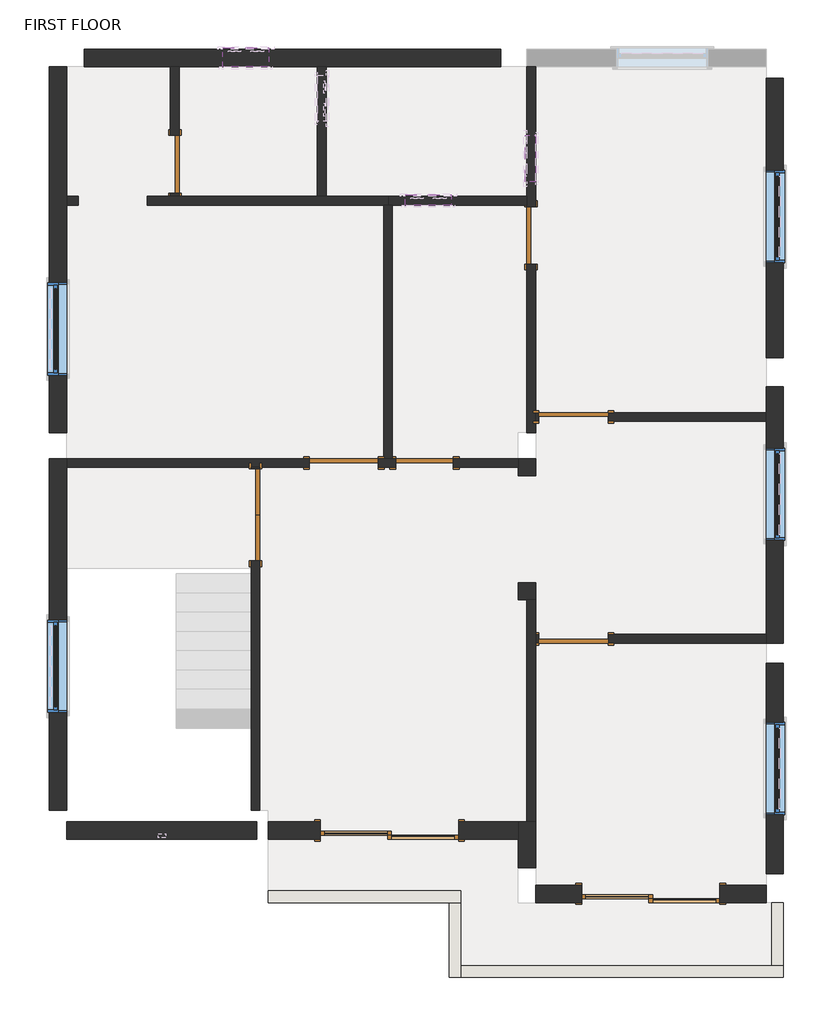
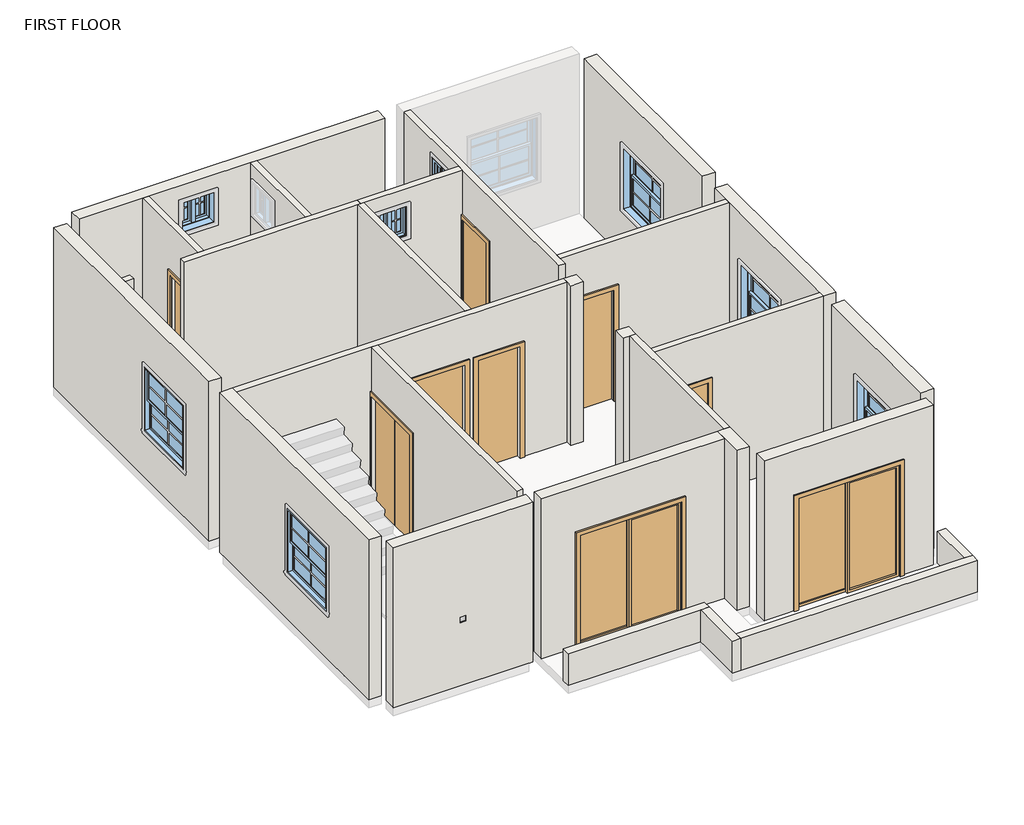
# One storey, part 1 of 2: 28 walls, 9 doors, 8 windows.
"""IFC4 building model written with IfcOpenShell, lengths in millimetres."""

from ifc_helpers import new_model, si_unit, frame, origin, place, context, project, spatial, polyline, outline, extrude, faceted_brep, transform, mapped, element, save
from components import door_double_flush_panel_4_x7_eb8a45e1, door_d4d75d1e, door_78caadf7, door_214872d5, single_flush_3_x7_e5f9f3c4, single_flush_3_x7_305aa2a5, window_casement_double_2_x2_e4709907, window_casement_double_2_x2_3fc3773f, window_double_hung_4_x4_ec8efb0e

model = new_model("IFC4")

# Units and contexts
model_context = context("Model", 3, world=origin())
ifc_project = project(units=[si_unit("LENGTHUNIT", "METRE", prefix="MILLI")], contexts=[model_context])

# Site, building, storey
site = spatial("IfcSite", under=ifc_project)
building = spatial("IfcBuilding", under=site)
storey = spatial("IfcBuildingStorey", under=building, Name="FIRST FLOOR", Elevation=3200.4)

# Doors
placement = place(None, origin())
door_double_flush_panel_4_x7_shape = door_double_flush_panel_4_x7_eb8a45e1(model_context)
element("IfcDoor", 1, ObjectType="Door-Double-Flush_Panel : 4'X7'", at=placement, inside=storey, context=model_context, shape_type="MappedRepresentation", body=[
    mapped(door_double_flush_panel_4_x7_shape, transform((-10167.2709734, 2734.5670657, 3200.4), x_axis=(0.0, -1.0, 0.0), y_axis=(1.0, 0.0, 0.0), z_axis=(0.0, 0.0, 1.0))),
])
door_shape = door_d4d75d1e(model_context)
element("IfcDoor", 2, ObjectType="Door-Double-Sliding : 72\" x 84\"", at=placement, inside=storey, context=model_context, shape_type="MappedRepresentation", body=[
    mapped(door_shape, transform((-4941.2209734, -2148.5829343, 3200.4), x_axis=(-1.0, 0.0, 0.0), y_axis=(0.0, -1.0, 0.0), z_axis=(0.0, 0.0, 1.0))),
])
element("IfcDoor", 3, ObjectType="Door-Double-Sliding : 72\" x 84\"", at=placement, inside=storey, context=model_context, shape_type="MappedRepresentation", body=[
    mapped(door_shape, transform((-8395.6209734, -1310.3829343, 3200.4), x_axis=(-1.0, 0.0, 0.0), y_axis=(0.0, -1.0, 0.0), z_axis=(0.0, 0.0, 1.0))),
])
door_2_shape = door_78caadf7(model_context)
element("IfcDoor", 4, ObjectType="Single-Flush : 2'6\"", at=placement, inside=storey, context=model_context, shape_type="MappedRepresentation", body=[
    mapped(door_2_shape, transform((-7932.0709734, 3420.3670657, 3200.4), x_axis=(-1.0, 0.0, 0.0), y_axis=(0.0, -1.0, 0.0), z_axis=(0.0, 0.0, 1.0))),
])
door_3_shape = door_214872d5(model_context)
element("IfcDoor", 5, ObjectType="Single-Flush : 2'6\"", at=placement, inside=storey, context=model_context, shape_type="MappedRepresentation", body=[
    mapped(door_3_shape, transform((-11234.0709734, 7370.0670657, 3200.4), x_axis=(0.0, -1.0, 0.0), y_axis=(1.0, 0.0, 0.0), z_axis=(0.0, 0.0, 1.0))),
])
element("IfcDoor", 6, ObjectType="Single-Flush : 2'6\"", at=placement, inside=storey, context=model_context, shape_type="MappedRepresentation", body=[
    mapped(door_3_shape, transform((-6522.3709734, 6430.2670657, 3200.4), x_axis=(0.0, 1.0, 0.0), y_axis=(-1.0, 0.0, 0.0), z_axis=(0.0, 0.0, 1.0))),
])
single_flush_3_x7_shape = single_flush_3_x7_e5f9f3c4(model_context)
element("IfcDoor", 7, ObjectType="Single-Flush : 3'X7'", at=placement, inside=storey, context=model_context, shape_type="MappedRepresentation", body=[
    mapped(single_flush_3_x7_shape, transform((-8998.8709734, 3420.3670657, 3200.4), x_axis=(1.0, 0.0, 0.0), y_axis=(0.0, 1.0, 0.0), z_axis=(0.0, 0.0, 1.0))),
])
element("IfcDoor", 8, ObjectType="Single-Flush : 3'X7'", at=placement, inside=storey, context=model_context, shape_type="MappedRepresentation", body=[
    mapped(single_flush_3_x7_shape, transform((-5963.5709734, 1096.2670657, 3200.4), x_axis=(-1.0, 0.0, 0.0), y_axis=(0.0, -1.0, 0.0), z_axis=(0.0, 0.0, 1.0))),
])
single_flush_3_x7_2_shape = single_flush_3_x7_305aa2a5(model_context)
element("IfcDoor", 9, ObjectType="Single-Flush : 3'X7'", at=placement, inside=storey, context=model_context, shape_type="MappedRepresentation", body=[
    mapped(single_flush_3_x7_2_shape, transform((-5963.5709734, 4029.9670657, 3200.4), x_axis=(-1.0, 0.0, 0.0), y_axis=(0.0, -1.0, 0.0), z_axis=(0.0, 0.0, 1.0))),
])

# Walls
element("IfcWall", 10, ObjectType="4.5\"", at=placement, inside=storey, context=model_context, shape_type="SweptSolid", body=[
    extrude(outline(polyline([(6989.0670657, 5334.0), (6989.0670657, 3200.4), (6944.6170657, 3200.4), (6944.6170657, 6248.4), (8659.1170657, 6248.4), (8659.1170657, 3200.4), (7751.0670657, 3200.4), (7751.0670657, 5334.0), (6989.0670657, 5334.0)])), frame((-11291.2209734, 0.0, 0.0), z_axis=(1.0, 0.0, 0.0), x_axis=(0.0, 1.0, 0.0)), (0.0, 0.0, 1.0), 114.3),
])
element("IfcWall", 11, ObjectType="4.5\"", at=placement, inside=storey, context=model_context, shape_type="SweptSolid", body=[
    extrude(outline(polyline([(-12510.4209734, 6830.3170657), (-12662.8209734, 6830.3170657), (-12662.8209734, 6944.6170657), (-12510.4209734, 6944.6170657), (-12510.4209734, 6830.3170657)])), frame((0.0, 0.0, 3200.4), z_axis=(0.0, 0.0, 1.0), x_axis=(1.0, 0.0, 0.0)), (0.0, 0.0, 1.0), 3048.0),
])
element("IfcWall", 12, ObjectType="4.5\"", at=placement, inside=storey, context=model_context, shape_type="Brep", body=[
    faceted_brep([(-11596.0209734, 6830.3170657, 3200.4), (-8471.8209734, 6830.3170657, 3200.4), (-8414.6709734, 6830.3170657, 3200.4), (-8414.6709734, 6830.3170657, 6248.4), (-8471.8209734, 6830.3170657, 6248.4), (-11596.0209734, 6830.3170657, 6248.4), (-11596.0209734, 6944.6170657, 3200.4), (-11596.0209734, 6944.6170657, 6248.4), (-11291.2209734, 6944.6170657, 6248.4), (-11176.9209734, 6944.6170657, 6248.4), (-9348.1209734, 6944.6170657, 6248.4), (-9233.8209734, 6944.6170657, 6248.4), (-8414.6709734, 6944.6170657, 6248.4), (-8414.6709734, 6944.6170657, 3200.4), (-9233.8209734, 6944.6170657, 3200.4), (-9348.1209734, 6944.6170657, 3200.4), (-11176.9209734, 6944.6170657, 3200.4), (-11291.2209734, 6944.6170657, 3200.4)], [[[0, 1, 2, 3, 4, 5]], [[6, 7, 8, 9, 10, 11, 12, 13, 14, 15, 16, 17]], [[2, 1, 0, 6, 17, 16, 15, 14, 13]], [[3, 2, 13, 12]], [[5, 4, 3, 12, 11, 10, 9, 8, 7]], [[0, 5, 7, 6]]]),
])
element("IfcWall", 13, ObjectType="4.5\"", at=placement, inside=storey, context=model_context, shape_type="SweptSolid", body=[
    extrude(outline(polyline([(8659.1170657, 3200.4), (6944.6170657, 3200.4), (6944.6170657, 6248.4), (8659.1170657, 6248.4), (8659.1170657, 3200.4)]), holes=[polyline([(7935.2170657, 5943.6), (7935.2170657, 5334.0), (8544.8170657, 5334.0), (8544.8170657, 5943.6), (7935.2170657, 5943.6)])]), frame((-9348.1209734, 0.0, 0.0), z_axis=(1.0, 0.0, 0.0), x_axis=(0.0, 1.0, 0.0)), (0.0, 0.0, 1.0), 114.3),
])
element("IfcWall", 14, ObjectType="4.5\"", at=placement, inside=storey, context=model_context, shape_type="Brep", body=[
    faceted_brep([(-6579.5209734, 8659.1170657, 3200.4), (-6579.5209734, 6944.6170657, 3200.4), (-6579.5209734, 6830.3170657, 3200.4), (-6579.5209734, 6811.2670657, 3200.4), (-6579.5209734, 6811.2670657, 5334.0), (-6579.5209734, 6049.2670657, 5334.0), (-6579.5209734, 6049.2670657, 3200.4), (-6579.5209734, 3820.4170657, 3200.4), (-6579.5209734, 3820.4170657, 6248.4), (-6579.5209734, 6830.3170657, 6248.4), (-6579.5209734, 6944.6170657, 6248.4), (-6579.5209734, 8659.1170657, 6248.4), (-6579.5209734, 7751.0670657, 5943.6), (-6579.5209734, 7141.4670657, 5943.6), (-6579.5209734, 7141.4670657, 5334.0), (-6579.5209734, 7751.0670657, 5334.0), (-6465.2209734, 6811.2670657, 5334.0), (-6465.2209734, 6811.2670657, 3200.4), (-6465.2209734, 8659.1170657, 3200.4), (-6465.2209734, 8659.1170657, 6248.4), (-6465.2209734, 4087.1170657, 6248.4), (-6465.2209734, 3972.8170657, 6248.4), (-6465.2209734, 3820.4170657, 6248.4), (-6465.2209734, 3820.4170657, 3200.4), (-6465.2209734, 3972.8170657, 3200.4), (-6465.2209734, 4087.1170657, 3200.4), (-6465.2209734, 6049.2670657, 3200.4), (-6465.2209734, 6049.2670657, 5334.0), (-6465.2209734, 7751.0670657, 5943.6), (-6465.2209734, 7751.0670657, 5334.0), (-6465.2209734, 7141.4670657, 5334.0), (-6465.2209734, 7141.4670657, 5943.6)], [[[0, 1, 2, 3, 4, 5, 6, 7, 8, 9, 10, 11], [12, 13, 14, 15]], [[16, 17, 18, 19, 20, 21, 22, 23, 24, 25, 26, 27], [28, 29, 30, 31]], [[18, 17, 3, 2, 1, 0]], [[26, 25, 24, 23, 7, 6]], [[8, 7, 23, 22]], [[11, 10, 9, 8, 22, 21, 20, 19]], [[0, 11, 19, 18]], [[4, 3, 17, 16]], [[5, 4, 16, 27]], [[6, 5, 27, 26]], [[29, 28, 12, 15]], [[30, 29, 15, 14]], [[31, 30, 14, 13]], [[28, 31, 13, 12]]]),
])
element("IfcWall", 15, ObjectType="4.5\"", at=placement, inside=storey, context=model_context, shape_type="Brep", body=[
    faceted_brep([(-6579.5209734, 6944.6170657, 3200.4), (-8414.6709734, 6944.6170657, 3200.4), (-8414.6709734, 6944.6170657, 6248.4), (-6579.5209734, 6944.6170657, 6248.4), (-7576.4709734, 6944.6170657, 5943.6), (-8186.0709734, 6944.6170657, 5943.6), (-8186.0709734, 6944.6170657, 5334.0), (-7576.4709734, 6944.6170657, 5334.0), (-6579.5209734, 6830.3170657, 3200.4), (-6579.5209734, 6830.3170657, 6248.4), (-8357.5209734, 6830.3170657, 6248.4), (-8414.6709734, 6830.3170657, 6248.4), (-8414.6709734, 6830.3170657, 3200.4), (-8357.5209734, 6830.3170657, 3200.4), (-7576.4709734, 6830.3170657, 5943.6), (-7576.4709734, 6830.3170657, 5334.0), (-8186.0709734, 6830.3170657, 5334.0), (-8186.0709734, 6830.3170657, 5943.6)], [[[0, 1, 2, 3], [4, 5, 6, 7]], [[8, 9, 10, 11, 12, 13], [14, 15, 16, 17]], [[1, 0, 8, 13, 12]], [[2, 1, 12, 11]], [[3, 2, 11, 10, 9]], [[0, 3, 9, 8]], [[15, 14, 4, 7]], [[16, 15, 7, 6]], [[17, 16, 6, 5]], [[14, 17, 5, 4]]]),
])
element("IfcWall", 16, ObjectType="4.5\"", at=placement, inside=storey, context=model_context, shape_type="Brep", body=[
    faceted_brep([(-8471.8209734, 6830.3170657, 3200.4), (-8471.8209734, 3477.5170657, 3200.4), (-8471.8209734, 3477.5170657, 6248.4), (-8471.8209734, 6830.3170657, 6248.4), (-8357.5209734, 6830.3170657, 3200.4), (-8357.5209734, 6830.3170657, 6248.4), (-8357.5209734, 3477.5170657, 6248.4), (-8357.5209734, 3477.5170657, 3200.4), (-8414.6709734, 6830.3170657, 3200.4), (-8414.6709734, 6830.3170657, 6248.4)], [[[0, 1, 2, 3]], [[4, 5, 6, 7]], [[1, 0, 8, 4, 7]], [[3, 2, 6, 5, 9]], [[0, 3, 9, 5, 4, 8]], [[2, 1, 7, 6]]]),
])
element("IfcWall", 17, ObjectType="4.5\"", at=placement, inside=storey, context=model_context, shape_type="Brep", body=[
    faceted_brep([(-8313.0709734, 3477.5170657, 5334.0), (-8313.0709734, 3477.5170657, 3200.4), (-8357.5209734, 3477.5170657, 3200.4), (-8471.8209734, 3477.5170657, 3200.4), (-8541.6709734, 3477.5170657, 3200.4), (-8541.6709734, 3477.5170657, 5334.0), (-9456.0709734, 3477.5170657, 5334.0), (-9456.0709734, 3477.5170657, 3200.4), (-12662.8209734, 3477.5170657, 3200.4), (-12662.8209734, 3477.5170657, 6248.4), (-8471.8209734, 3477.5170657, 6248.4), (-8357.5209734, 3477.5170657, 6248.4), (-6693.8209734, 3477.5170657, 6248.4), (-6693.8209734, 3477.5170657, 3200.4), (-7551.0709734, 3477.5170657, 3200.4), (-7551.0709734, 3477.5170657, 5334.0), (-8541.6709734, 3363.2170657, 3200.4), (-8313.0709734, 3363.2170657, 3200.4), (-8313.0709734, 3363.2170657, 5334.0), (-7551.0709734, 3363.2170657, 5334.0), (-7551.0709734, 3363.2170657, 3200.4), (-6693.8209734, 3363.2170657, 3200.4), (-6693.8209734, 3363.2170657, 6248.4), (-10110.1209734, 3363.2170657, 6248.4), (-10224.4209734, 3363.2170657, 6248.4), (-12662.8209734, 3363.2170657, 6248.4), (-12662.8209734, 3363.2170657, 3200.4), (-10224.4209734, 3363.2170657, 3200.4), (-10110.1209734, 3363.2170657, 3200.4), (-9456.0709734, 3363.2170657, 3200.4), (-9456.0709734, 3363.2170657, 5334.0), (-8541.6709734, 3363.2170657, 5334.0)], [[[0, 1, 2, 3, 4, 5, 6, 7, 8, 9, 10, 11, 12, 13, 14, 15]], [[16, 17, 18, 19, 20, 21, 22, 23, 24, 25, 26, 27, 28, 29, 30, 31]], [[29, 28, 27, 26, 8, 7]], [[14, 13, 21, 20]], [[4, 3, 2, 1, 17, 16]], [[12, 11, 10, 9, 25, 24, 23, 22]], [[9, 8, 26, 25]], [[13, 12, 22, 21]], [[5, 4, 16, 31]], [[6, 5, 31, 30]], [[7, 6, 30, 29]], [[18, 17, 1, 0]], [[19, 18, 0, 15]], [[20, 19, 15, 14]]]),
])
element("IfcWall", 18, ObjectType="4.5\"", at=placement, inside=storey, context=model_context, shape_type="SweptSolid", body=[
    extrude(outline(polyline([(-1170.6829343, 3200.4), (-1170.6829343, 6248.4), (3363.2170657, 6248.4), (3363.2170657, 3200.4), (3344.1670657, 3200.4), (3344.1670657, 5334.0), (2124.9670657, 5334.0), (2124.9670657, 3200.4), (-1170.6829343, 3200.4)])), frame((-10224.4209734, 0.0, 0.0), z_axis=(1.0, 0.0, 0.0), x_axis=(0.0, 1.0, 0.0)), (0.0, 0.0, 1.0), 114.3),
])
element("IfcWall", 19, ObjectType="4.5\"", at=placement, inside=storey, context=model_context, shape_type="SweptSolid", body=[
    extrude(outline(polyline([(3200.4, -6465.2209734), (3200.4, -6420.7709734), (5334.0, -6420.7709734), (5334.0, -5506.3709734), (3200.4, -5506.3709734), (3200.4, -3417.2209734), (6248.4, -3417.2209734), (6248.4, -6465.2209734), (3200.4, -6465.2209734)])), frame((0.0, 3972.8170657, 0.0), z_axis=(0.0, 1.0, 0.0), x_axis=(0.0, 0.0, 1.0)), (0.0, 0.0, 1.0), 114.3),
])
element("IfcWall", 20, ObjectType="4.5\"", at=placement, inside=storey, context=model_context, shape_type="SweptSolid", body=[
    extrude(outline(polyline([(3200.4, -6465.2209734), (3200.4, -6420.7709734), (5334.0, -6420.7709734), (5334.0, -5506.3709734), (3200.4, -5506.3709734), (3200.4, -3417.2209734), (6248.4, -3417.2209734), (6248.4, -6465.2209734), (3200.4, -6465.2209734)])), frame((0.0, 1039.1170657, 0.0), z_axis=(0.0, 1.0, 0.0), x_axis=(0.0, 0.0, 1.0)), (0.0, 0.0, 1.0), 114.3),
])
element("IfcWall", 21, ObjectType="4.5\"", at=placement, inside=storey, context=model_context, shape_type="Brep", body=[
    faceted_brep([(-6579.5209734, 1610.6170657, 3200.4), (-6579.5209734, -1323.0829343, 3200.4), (-6579.5209734, -1323.0829343, 6248.4), (-6579.5209734, 1610.6170657, 6248.4), (-6465.2209734, 1610.6170657, 3200.4), (-6465.2209734, 1610.6170657, 6248.4), (-6465.2209734, 1153.4170657, 6248.4), (-6465.2209734, 1039.1170657, 6248.4), (-6465.2209734, -1323.0829343, 6248.4), (-6465.2209734, -1323.0829343, 3200.4), (-6465.2209734, 1039.1170657, 3200.4), (-6465.2209734, 1153.4170657, 3200.4)], [[[0, 1, 2, 3]], [[4, 5, 6, 7, 8, 9, 10, 11]], [[1, 0, 4, 11, 10, 9]], [[3, 2, 8, 7, 6, 5]], [[0, 3, 5, 4]], [[2, 1, 9, 8]]]),
])
element("IfcWall", 22, ObjectType="6\"", at=placement, inside=storey, context=model_context, shape_type="Brep", body=[
    faceted_brep([(-9995.8209734, -2389.8829343, 3200.4), (-7608.2209734, -2389.8829343, 3200.4), (-7455.8209734, -2389.8829343, 3200.4), (-7455.8209734, -2389.8829343, 3810.0), (-7608.2209734, -2389.8829343, 3810.0), (-9995.8209734, -2389.8829343, 3810.0), (-9995.8209734, -2237.4829343, 3200.4), (-9995.8209734, -2237.4829343, 3810.0), (-7455.8209734, -2237.4829343, 3810.0), (-7455.8209734, -2237.4829343, 3200.4)], [[[0, 1, 2, 3, 4, 5]], [[6, 7, 8, 9]], [[2, 1, 0, 6, 9]], [[5, 4, 3, 8, 7]], [[0, 5, 7, 6]], [[3, 2, 9, 8]]]),
])
element("IfcWall", 23, ObjectType="6\"", at=placement, inside=storey, context=model_context, shape_type="Brep", body=[
    faceted_brep([(-7608.2209734, -2389.8829343, 3200.4), (-7608.2209734, -3380.4829343, 3200.4), (-7608.2209734, -3380.4829343, 3810.0), (-7608.2209734, -2389.8829343, 3810.0), (-7455.8209734, -2389.8829343, 3200.4), (-7455.8209734, -2389.8829343, 3810.0), (-7455.8209734, -3228.0829343, 3810.0), (-7455.8209734, -3380.4829343, 3810.0), (-7455.8209734, -3380.4829343, 3200.4), (-7455.8209734, -3228.0829343, 3200.4)], [[[0, 1, 2, 3]], [[4, 5, 6, 7, 8, 9]], [[1, 0, 4, 9, 8]], [[3, 2, 7, 6, 5]], [[0, 3, 5, 4]], [[2, 1, 8, 7]]]),
])
element("IfcWall", 24, ObjectType="6\"", at=placement, inside=storey, context=model_context, shape_type="Brep", body=[
    faceted_brep([(-7455.8209734, -3380.4829343, 3200.4), (-3188.6209734, -3380.4829343, 3200.4), (-3188.6209734, -3380.4829343, 3810.0), (-7455.8209734, -3380.4829343, 3810.0), (-7455.8209734, -3228.0829343, 3200.4), (-7455.8209734, -3228.0829343, 3810.0), (-3341.0209734, -3228.0829343, 3810.0), (-3188.6209734, -3228.0829343, 3810.0), (-3188.6209734, -3228.0829343, 3200.4), (-3341.0209734, -3228.0829343, 3200.4)], [[[0, 1, 2, 3]], [[4, 5, 6, 7, 8, 9]], [[1, 0, 4, 9, 8]], [[3, 2, 7, 6, 5]], [[0, 3, 5, 4]], [[2, 1, 8, 7]]]),
])
element("IfcWall", 25, ObjectType="6\"", at=placement, inside=storey, context=model_context, shape_type="SweptSolid", body=[
    extrude(outline(polyline([(-3188.6209734, -2389.8829343), (-3188.6209734, -3228.0829343), (-3341.0209734, -3228.0829343), (-3341.0209734, -2389.8829343), (-3188.6209734, -2389.8829343)])), frame((0.0, 0.0, 3200.4), z_axis=(0.0, 0.0, 1.0), x_axis=(1.0, 0.0, 0.0)), (0.0, 0.0, 1.0), 609.6),
])
element("IfcWall", 26, ObjectType="9\"", at=placement, inside=storey, context=model_context, shape_type="Brep", body=[
    faceted_brep([(-12891.4209734, 8659.1170657, 3200.4), (-12891.4209734, 3820.4170657, 3200.4), (-12891.4209734, 3820.4170657, 6248.4), (-12891.4209734, 8659.1170657, 6248.4), (-12891.4209734, 4582.4170657, 5334.0), (-12891.4209734, 4582.4170657, 4114.8), (-12891.4209734, 5801.6170657, 4114.8), (-12891.4209734, 5801.6170657, 5334.0), (-12662.8209734, 8659.1170657, 3200.4), (-12662.8209734, 8659.1170657, 6248.4), (-12662.8209734, 6944.6170657, 6248.4), (-12662.8209734, 6830.3170657, 6248.4), (-12662.8209734, 3820.4170657, 6248.4), (-12662.8209734, 3820.4170657, 3200.4), (-12662.8209734, 6830.3170657, 3200.4), (-12662.8209734, 6944.6170657, 3200.4), (-12662.8209734, 4582.4170657, 5334.0), (-12662.8209734, 5801.6170657, 5334.0), (-12662.8209734, 5801.6170657, 4114.8), (-12662.8209734, 4582.4170657, 4114.8)], [[[0, 1, 2, 3], [4, 5, 6, 7]], [[8, 9, 10, 11, 12, 13, 14, 15], [16, 17, 18, 19]], [[1, 0, 8, 15, 14, 13]], [[2, 1, 13, 12]], [[3, 2, 12, 11, 10, 9]], [[0, 3, 9, 8]], [[5, 4, 16, 19]], [[6, 5, 19, 18]], [[7, 6, 18, 17]], [[4, 7, 17, 16]]]),
])
element("IfcWall", 27, ObjectType="9\"", at=placement, inside=storey, context=model_context, shape_type="Brep", body=[
    faceted_brep([(-12891.4209734, 3477.5170657, 3200.4), (-12891.4209734, 3363.2170657, 3200.4), (-12891.4209734, -1170.6829343, 3200.4), (-12891.4209734, -1170.6829343, 6248.4), (-12891.4209734, 3363.2170657, 6248.4), (-12891.4209734, 3477.5170657, 6248.4), (-12891.4209734, 124.7170657, 5334.0), (-12891.4209734, 124.7170657, 4114.8), (-12891.4209734, 1343.9170657, 4114.8), (-12891.4209734, 1343.9170657, 5334.0), (-12662.8209734, 3477.5170657, 3200.4), (-12662.8209734, 3477.5170657, 6248.4), (-12662.8209734, 3363.2170657, 6248.4), (-12662.8209734, -1170.6829343, 6248.4), (-12662.8209734, -1170.6829343, 3200.4), (-12662.8209734, 3363.2170657, 3200.4), (-12662.8209734, 124.7170657, 5334.0), (-12662.8209734, 1343.9170657, 5334.0), (-12662.8209734, 1343.9170657, 4114.8), (-12662.8209734, 124.7170657, 4114.8)], [[[0, 1, 2, 3, 4, 5], [6, 7, 8, 9]], [[10, 11, 12, 13, 14, 15], [16, 17, 18, 19]], [[2, 1, 0, 10, 15, 14]], [[3, 2, 14, 13]], [[5, 4, 3, 13, 12, 11]], [[0, 5, 11, 10]], [[7, 6, 16, 19]], [[8, 7, 19, 18]], [[9, 8, 18, 17]], [[6, 9, 17, 16]]]),
])
element("IfcWall", 28, ObjectType="9\"", at=placement, inside=storey, context=model_context, shape_type="Brep", body=[
    faceted_brep([(-12434.2209734, 8659.1170657, 3200.4), (-11291.2209734, 8659.1170657, 3200.4), (-11176.9209734, 8659.1170657, 3200.4), (-9348.1209734, 8659.1170657, 3200.4), (-9233.8209734, 8659.1170657, 3200.4), (-6922.4209734, 8659.1170657, 3200.4), (-6922.4209734, 8659.1170657, 6248.4), (-9233.8209734, 8659.1170657, 6248.4), (-9348.1209734, 8659.1170657, 6248.4), (-11176.9209734, 8659.1170657, 6248.4), (-11291.2209734, 8659.1170657, 6248.4), (-12434.2209734, 8659.1170657, 6248.4), (-9989.4709734, 8659.1170657, 5943.6), (-9989.4709734, 8659.1170657, 5334.0), (-10599.0709734, 8659.1170657, 5334.0), (-10599.0709734, 8659.1170657, 5943.6), (-12434.2209734, 8887.7170657, 3200.4), (-12434.2209734, 8887.7170657, 6248.4), (-6922.4209734, 8887.7170657, 6248.4), (-6922.4209734, 8887.7170657, 3200.4), (-9989.4709734, 8887.7170657, 5943.6), (-10599.0709734, 8887.7170657, 5943.6), (-10599.0709734, 8887.7170657, 5334.0), (-9989.4709734, 8887.7170657, 5334.0)], [[[0, 1, 2, 3, 4, 5, 6, 7, 8, 9, 10, 11], [12, 13, 14, 15]], [[16, 17, 18, 19], [20, 21, 22, 23]], [[5, 4, 3, 2, 1, 0, 16, 19]], [[6, 5, 19, 18]], [[11, 10, 9, 8, 7, 6, 18, 17]], [[0, 11, 17, 16]], [[13, 12, 20, 23]], [[14, 13, 23, 22]], [[15, 14, 22, 21]], [[12, 15, 21, 20]]]),
])
element("IfcWall", 29, ObjectType="9\"", at=placement, inside=storey, context=model_context, shape_type="SweptSolid", body=[
    extrude(outline(polyline([(8506.7170657, 3200.4), (4811.0170657, 3200.4), (4811.0170657, 6248.4), (8506.7170657, 6248.4), (8506.7170657, 3200.4)]), holes=[polyline([(7287.5170657, 5334.0), (6068.3170657, 5334.0), (6068.3170657, 4114.8), (7287.5170657, 4114.8), (7287.5170657, 5334.0)])]), frame((-3417.2209734, 0.0, 0.0), z_axis=(1.0, 0.0, 0.0), x_axis=(0.0, 1.0, 0.0)), (0.0, 0.0, 1.0), 228.6),
])
element("IfcWall", 30, ObjectType="9\"", at=placement, inside=storey, context=model_context, shape_type="Brep", body=[
    faceted_brep([(-3417.2209734, 4430.0170657, 3200.4), (-3417.2209734, 4087.1170657, 3200.4), (-3417.2209734, 3972.8170657, 3200.4), (-3417.2209734, 1153.4170657, 3200.4), (-3417.2209734, 1039.1170657, 3200.4), (-3417.2209734, 1039.1170657, 6248.4), (-3417.2209734, 1153.4170657, 6248.4), (-3417.2209734, 3972.8170657, 6248.4), (-3417.2209734, 4087.1170657, 6248.4), (-3417.2209734, 4430.0170657, 6248.4), (-3417.2209734, 3617.2170657, 5334.0), (-3417.2209734, 2398.0170657, 5334.0), (-3417.2209734, 2398.0170657, 4114.8), (-3417.2209734, 3617.2170657, 4114.8), (-3188.6209734, 4430.0170657, 3200.4), (-3188.6209734, 4430.0170657, 6248.4), (-3188.6209734, 1153.4170657, 6248.4), (-3188.6209734, 1039.1170657, 6248.4), (-3188.6209734, 1039.1170657, 3200.4), (-3188.6209734, 1153.4170657, 3200.4), (-3188.6209734, 3617.2170657, 5334.0), (-3188.6209734, 3617.2170657, 4114.8), (-3188.6209734, 2398.0170657, 4114.8), (-3188.6209734, 2398.0170657, 5334.0)], [[[0, 1, 2, 3, 4, 5, 6, 7, 8, 9], [10, 11, 12, 13]], [[14, 15, 16, 17, 18, 19], [20, 21, 22, 23]], [[4, 3, 2, 1, 0, 14, 19, 18]], [[9, 8, 7, 6, 5, 17, 16, 15]], [[0, 9, 15, 14]], [[5, 4, 18, 17]], [[21, 20, 10, 13]], [[22, 21, 13, 12]], [[23, 22, 12, 11]], [[20, 23, 11, 10]]]),
])
element("IfcWall", 31, ObjectType="9\"", at=placement, inside=storey, context=model_context, shape_type="SweptSolid", body=[
    extrude(outline(polyline([(772.4170657, 3200.4), (-2008.8829343, 3200.4), (-2008.8829343, 6248.4), (772.4170657, 6248.4), (772.4170657, 3200.4)]), holes=[polyline([(-8.6329343, 5334.0), (-1227.8329343, 5334.0), (-1227.8329343, 4114.8), (-8.6329343, 4114.8), (-8.6329343, 5334.0)])]), frame((-3417.2209734, 0.0, 0.0), z_axis=(1.0, 0.0, 0.0), x_axis=(0.0, 1.0, 0.0)), (0.0, 0.0, 1.0), 228.6),
])
element("IfcWall", 32, ObjectType="9\"", at=placement, inside=storey, context=model_context, shape_type="SweptSolid", body=[
    extrude(outline(polyline([(3200.4, -6465.2209734), (3200.4, -5855.6209734), (5334.0, -5855.6209734), (5334.0, -4026.8209734), (3200.4, -4026.8209734), (3200.4, -3417.2209734), (6248.4, -3417.2209734), (6248.4, -6465.2209734), (3200.4, -6465.2209734)])), frame((0.0, -2389.8829343, 0.0), z_axis=(0.0, 1.0, 0.0), x_axis=(0.0, 0.0, 1.0)), (0.0, 0.0, 1.0), 228.6),
])
element("IfcWall", 33, ObjectType="9\"", at=placement, inside=storey, context=model_context, shape_type="Brep", body=[
    faceted_brep([(-6465.2209734, -1932.6829343, 3200.4), (-6465.2209734, -1323.0829343, 3200.4), (-6465.2209734, -1323.0829343, 6248.4), (-6465.2209734, -1932.6829343, 6248.4), (-6693.8209734, -1932.6829343, 3200.4), (-6693.8209734, -1932.6829343, 6248.4), (-6693.8209734, -1551.6829343, 6248.4), (-6693.8209734, -1323.0829343, 6248.4), (-6693.8209734, -1323.0829343, 3200.4), (-6693.8209734, -1551.6829343, 3200.4), (-6579.5209734, -1323.0829343, 3200.4), (-6579.5209734, -1323.0829343, 6248.4)], [[[0, 1, 2, 3]], [[4, 5, 6, 7, 8, 9]], [[1, 0, 4, 9, 8, 10]], [[3, 2, 11, 7, 6, 5]], [[0, 3, 5, 4]], [[2, 1, 10, 8, 7, 11]]]),
])
element("IfcWall", 34, ObjectType="9\"", at=placement, inside=storey, context=model_context, shape_type="SweptSolid", body=[
    extrude(outline(polyline([(3200.4, -9995.8209734), (3200.4, -9310.0209734), (5334.0, -9310.0209734), (5334.0, -7481.2209734), (3200.4, -7481.2209734), (3200.4, -6693.8209734), (6248.4, -6693.8209734), (6248.4, -9995.8209734), (3200.4, -9995.8209734)])), frame((0.0, -1551.6829343, 0.0), z_axis=(0.0, 1.0, 0.0), x_axis=(0.0, 0.0, 1.0)), (0.0, 0.0, 1.0), 228.6),
])
element("IfcWall", 35, ObjectType="9\"", at=placement, inside=storey, context=model_context, shape_type="Brep", body=[
    faceted_brep([(-10148.2209734, -1323.0829343, 3200.4), (-10224.4209734, -1323.0829343, 3200.4), (-12662.8209734, -1323.0829343, 3200.4), (-12662.8209734, -1323.0829343, 6248.4), (-10224.4209734, -1323.0829343, 6248.4), (-10148.2209734, -1323.0829343, 6248.4), (-11355.5209734, -1323.0829343, 4502.7878889), (-11455.5209734, -1323.0829343, 4502.7878889), (-11455.5209734, -1323.0829343, 4402.7878889), (-11355.5209734, -1323.0829343, 4402.7878889), (-10148.2209734, -1551.6829343, 3200.4), (-10148.2209734, -1551.6829343, 6248.4), (-10224.4209734, -1551.6829343, 6248.4), (-12662.8209734, -1551.6829343, 6248.4), (-12662.8209734, -1551.6829343, 3200.4), (-10224.4209734, -1551.6829343, 3200.4), (-11355.5209734, -1551.6829343, 4502.7878889), (-11355.5209734, -1551.6829343, 4402.7878889), (-11455.5209734, -1551.6829343, 4402.7878889), (-11455.5209734, -1551.6829343, 4502.7878889)], [[[0, 1, 2, 3, 4, 5], [6, 7, 8, 9]], [[10, 11, 12, 13, 14, 15], [16, 17, 18, 19]], [[2, 1, 0, 10, 15, 14]], [[3, 2, 14, 13]], [[5, 4, 3, 13, 12, 11]], [[0, 5, 11, 10]], [[17, 16, 6, 9]], [[18, 17, 9, 8]], [[19, 18, 8, 7]], [[16, 19, 7, 6]]]),
])
element("IfcWall", 36, ObjectType="9\"", at=placement, inside=storey, context=model_context, shape_type="Brep", body=[
    faceted_brep([(-6693.8209734, 3477.5170657, 3200.4), (-6693.8209734, 3363.2170657, 3200.4), (-6693.8209734, 3248.9170657, 3200.4), (-6693.8209734, 3248.9170657, 6248.4), (-6693.8209734, 3363.2170657, 6248.4), (-6693.8209734, 3477.5170657, 6248.4), (-6465.2209734, 3477.5170657, 3200.4), (-6465.2209734, 3477.5170657, 6248.4), (-6465.2209734, 3363.2170657, 6248.4), (-6465.2209734, 3248.9170657, 6248.4), (-6465.2209734, 3248.9170657, 3200.4), (-6465.2209734, 3363.2170657, 3200.4)], [[[0, 1, 2, 3, 4, 5]], [[6, 7, 8, 9, 10, 11]], [[2, 1, 0, 6, 11, 10]], [[3, 2, 10, 9]], [[5, 4, 3, 9, 8, 7]], [[0, 5, 7, 6]]]),
])
element("IfcWall", 37, ObjectType="9\"", at=placement, inside=storey, context=model_context, shape_type="Brep", body=[
    faceted_brep([(-6693.8209734, 1839.2170657, 3200.4), (-6693.8209734, 1610.6170657, 3200.4), (-6693.8209734, 1610.6170657, 6248.4), (-6693.8209734, 1839.2170657, 6248.4), (-6465.2209734, 1839.2170657, 3200.4), (-6465.2209734, 1839.2170657, 6248.4), (-6465.2209734, 1610.6170657, 6248.4), (-6465.2209734, 1610.6170657, 3200.4), (-6579.5209734, 1610.6170657, 3200.4), (-6579.5209734, 1610.6170657, 6248.4)], [[[0, 1, 2, 3]], [[4, 5, 6, 7]], [[1, 0, 4, 7, 8]], [[2, 1, 8, 7, 6, 9]], [[3, 2, 9, 6, 5]], [[0, 3, 5, 4]]]),
])

# Windows
window_casement_double_2_x2_shape = window_casement_double_2_x2_e4709907(model_context)
element("IfcWindow", 38, ObjectType="Window-Casement-Double : 2'X2'", at=placement, inside=storey, context=model_context, shape_type="MappedRepresentation", body=[
    mapped(window_casement_double_2_x2_shape, transform((-7881.2709734, 6887.4670657, 4419.6), x_axis=(1.0, 0.0, 0.0), y_axis=(0.0, 1.0, 0.0), z_axis=(0.0, 0.0, 1.0))),
])
element("IfcWindow", 39, ObjectType="Window-Casement-Double : 2'X2'", at=placement, inside=storey, context=model_context, shape_type="MappedRepresentation", body=[
    mapped(window_casement_double_2_x2_shape, transform((-6522.3709734, 7446.2670657, 4419.6), x_axis=(0.0, 1.0, 0.0), y_axis=(-1.0, 0.0, 0.0), z_axis=(0.0, 0.0, 1.0))),
])
window_casement_double_2_x2_2_shape = window_casement_double_2_x2_3fc3773f(model_context)
element("IfcWindow", 40, ObjectType="Window-Casement-Double : 2'X2'", at=placement, inside=storey, context=model_context, shape_type="MappedRepresentation", body=[
    mapped(window_casement_double_2_x2_2_shape, transform((-10294.2709734, 8773.4170657, 4419.6), x_axis=(1.0, 0.0, 0.0), y_axis=(0.0, 1.0, 0.0), z_axis=(0.0, 0.0, 1.0))),
])
window_double_hung_4_x4_shape = window_double_hung_4_x4_ec8efb0e(model_context)
element("IfcWindow", 41, ObjectType="Window-Double-Hung : 4'X4'", at=placement, inside=storey, context=model_context, shape_type="MappedRepresentation", body=[
    mapped(window_double_hung_4_x4_shape, transform((-12777.1209734, 734.3170657, 3200.4), x_axis=(0.0, 1.0, 0.0), y_axis=(-1.0, 0.0, 0.0), z_axis=(0.0, 0.0, 1.0))),
])
element("IfcWindow", 42, ObjectType="Window-Double-Hung : 4'X4'", at=placement, inside=storey, context=model_context, shape_type="MappedRepresentation", body=[
    mapped(window_double_hung_4_x4_shape, transform((-12777.1209734, 5192.0170657, 3200.4), x_axis=(0.0, 1.0, 0.0), y_axis=(-1.0, 0.0, 0.0), z_axis=(0.0, 0.0, 1.0))),
])
element("IfcWindow", 43, ObjectType="Window-Double-Hung : 4'X4'", at=placement, inside=storey, context=model_context, shape_type="MappedRepresentation", body=[
    mapped(window_double_hung_4_x4_shape, transform((-3302.9209734, 6677.9170657, 3200.4), x_axis=(0.0, -1.0, 0.0), y_axis=(1.0, 0.0, 0.0), z_axis=(0.0, 0.0, 1.0))),
])
element("IfcWindow", 44, ObjectType="Window-Double-Hung : 4'X4'", at=placement, inside=storey, context=model_context, shape_type="MappedRepresentation", body=[
    mapped(window_double_hung_4_x4_shape, transform((-3302.9209734, 3007.6170657, 3200.4), x_axis=(0.0, -1.0, 0.0), y_axis=(1.0, 0.0, 0.0), z_axis=(0.0, 0.0, 1.0))),
])
element("IfcWindow", 45, ObjectType="Window-Double-Hung : 4'X4'", at=placement, inside=storey, context=model_context, shape_type="MappedRepresentation", body=[
    mapped(window_double_hung_4_x4_shape, transform((-3302.9209734, -618.2329343, 3200.4), x_axis=(0.0, -1.0, 0.0), y_axis=(1.0, 0.0, 0.0), z_axis=(0.0, 0.0, 1.0))),
])

save(model, "model.ifc")

# Revit data of these elements
# Type "Door-Double-Flush_Panel : 4'X7'"
#   Type Mark = "11"
#   Construction Type Id = "DOOR"
#   Assembly Code = "C1020"
#   Analytic Construction = "Wooden"
#   Thickness = 0' - 2"
#   Thermal Resistance (R) = 2.5876 (h·ft²·°F)/BTU
#   Swing Angle [instance default] = 90.00°
#   Panel Width = 2' - 0"
#   Heat Transfer Coefficient (U) = 0.3865 BTU/(h·ft²·°F)
#   Height = 7' - 0"
#   Trim Projection Ext = 0' - 1"
#   Trim Projection Int = 0' - 1"
#   Trim Width = 0' - 3"
#   Width = 4' - 0"
#   Define Thermal Properties by = 1
#   Panel Material = Wood - Birch - Solid Stained Light Low Gloss
#   Trim Material = Paint - Sienna
#   Visual Light Transmittance = 0
#   Solar Heat Gain Coefficient = 0
#   Function = (empty or 0)
#   Wall Closure = (empty or 0)
# Type "Door-Double-Sliding : 72\" x 84\""
#   Type Mark = "12"
#   Construction Type Id = "opn-d45"
#   Assembly Code = "C1020"
#   Analytic Construction = "Wood frame, double glass door "
#   Thickness = 0' - 2"
#   Thermal Resistance (R) = 1.8150 (h·ft²·°F)/BTU
#   Heat Transfer Coefficient (U) = 0.5510 BTU/(h·ft²·°F)
#   Height = 7' - 0"
#   Rail Width = 0' - 2"
#   Stiles = 0' - 2"
#   Trim Projection Ext = 0' - 1"
#   Trim Projection Int = 0' - 1"
#   Trim Width = 0' - 3"
#   Width = 6' - 0"
#   Define Thermal Properties by = 1
#   Glazing = Glass
#   Panel Material = Wood - Birch - Solid Stained Light Low Gloss
#   Trim Material = Paint - Sienna
#   Visual Light Transmittance = 0
#   Solar Heat Gain Coefficient = 0
#   Function = (empty or 0)
#   Wall Closure = (empty or 0)
# Type "Single-Flush : 2'6\""
#   Type Mark = "9"
#   Construction Type Id = "MDOOR"
#   Assembly Code = "C1020"
#   Analytic Construction = "Metal"
#   Thickness = 0' - 2"
#   Heat Transfer Coefficient (U) = 0.651978 BTU/(h·ft²·°F)
#   Height = 7' - 0"
#   Trim Projection Ext = 0' - 1"
#   Trim Projection Int = 0' - 1"
#   Trim Width = 0' - 3"
#   Width = 2' - 6"
#   Define Thermal Properties by = 1
#   Door Material = Door - Panel
#   Frame Material = Door - Frame
#   Visual Light Transmittance = 0
#   Solar Heat Gain Coefficient = 0
#   Function = (empty or 0)
#   Wall Closure = (empty or 0)
# Type "Single-Flush : 3'X7'"
#   Type Mark = "8"
#   Construction Type Id = "MDOOR"
#   Assembly Code = "C1020"
#   Analytic Construction = "Metal"
#   Thickness = 0' - 2"
#   Heat Transfer Coefficient (U) = 0.651978 BTU/(h·ft²·°F)
#   Height = 7' - 0"
#   Trim Projection Ext = 0' - 1"
#   Trim Projection Int = 0' - 1"
#   Trim Width = 0' - 3"
#   Width = 3' - 0"
#   Define Thermal Properties by = 1
#   Door Material = Door - Panel
#   Frame Material = Door - Frame
#   Visual Light Transmittance = 0
#   Solar Heat Gain Coefficient = 0
#   Function = (empty or 0)
#   Wall Closure = (empty or 0)
# Type "4.5\""
#   Assembly Code = "B2010"
#   Layers, outside or top first: 0' - 4 1/2" no material (function 1)
# Type "6\""
#   Assembly Code = "B2010"
#   Layers, outside or top first: 0' - 6" no material (function 1)
# Type "9\""
#   Assembly Code = "B2010"
#   Layers, outside or top first: 0' - 9" no material (function 1)
# Type "Window-Casement-Double : 2'X2'"
#   Type Mark = "20"
#   Fire Rating = "0.5h"
#   Assembly Code = "B2020100"
#   Analytic Construction = "Double glazing - domestic"
#   Frame Extension [instance default] = 0' - 0 1/4"
#   Window Inset [instance default] = 0' - 0"
#   Wall Thickness [instance default] = 0' - 6"
#   Interior Wall Closure [instance default] = 0' - 2 1/4"
#   Half Width = 1' - 0"
#   Visual Light Transmittance = 0.81
#   Thermal Resistance (R) = 1.8146 (h·ft²·°F)/BTU
#   Solar Heat Gain Coefficient = 0.76
#   Rough Width = 2' - 0 1/2"
#   Rough Height = 2' - 0 1/2"
#   Height = 2' - 0"
#   Heat Transfer Coefficient (U) = 0.5511 BTU/(h·ft²·°F)
#   Exterior Wall Closure [instance default] = 0' - 1 1/4"
#   Extension Jamb [instance default] = 0' - 2 1/4"
#   Default Sill Height = 3' - 0"
#   Width = 2' - 0"
#   Muntin Visibility = yes
#   Interior Trim Visibility [instance default] = yes
#   Exterior Trim Visibility [instance default] = yes
#   Extension Jamb Visibility [instance default] = yes
#   Interior Trim Material = Wood - Stained
#   Muntin Pattern = Muntin Pattern_2x2 : Muntin Pattern_2x2
#   Interior Trim = Trim-Window-Interior-Flat : Picture Frame
#   Interior Frame Material = Wood - Stained
#   Glass Panel Material = Glass
#   Exterior Trim Material = Clad - White
#   Exterior Trim = Trim-Window-Exterior-Flat : with Sill
#   Exterior Frame Material = Clad - White
#   Wall Closure = (empty or 0)
# Type "Window-Double-Hung : 4'X4'"
#   Type Mark = "19"
#   Fire Rating = "0.5h"
#   Construction Type Id = "DG-DR"
#   Assembly Code = "B2020100"
#   Analytic Construction = "Double glazing - domestic"
#   Wall Thickness [instance default] = 0' - 6"
#   Window Inset [instance default] = 0' - 0"
#   Visual Light Transmittance = 0.81
#   Thermal Resistance (R) = 1.8146 (h·ft²·°F)/BTU
#   Solar Heat Gain Coefficient = 0.76
#   Muntin Width = 3' - 6"
#   Muntin Height = 1' - 8 1/8"
#   Interior Wall Closure [instance default] = 0' - 1 1/2"
#   Rough Width = 4' - 0 1/2"
#   Rough Height = 4' - 0 1/2"
#   Frame Extension [instance default] = 0' - 1 1/4"
#   Exterior Wall Closure [instance default] = 0' - 0 1/2"
#   Extension Jamb [instance default] = 0' - 1 1/2"
#   Heat Transfer Coefficient (U) = 0.5511 BTU/(h·ft²·°F)
#   Height = 4' - 0"
#   Width = 4' - 0"
#   Top Muntin Visibility = yes
#   Indicator Visibility [instance default] = yes
#   Extension Jamb Visibility [instance default] = yes
#   Interior Trim Visibility [instance default] = yes
#   Exterior Trim Visibility [instance default] = yes
#   Define Thermal Properties by = 1
#   Bottom Muntin Visibility = yes
#   Muntin Pattern = Muntin Pattern_2x2 : Muntin Pattern_2x2
#   Interior Trim Material = Wood - Stained
#   Interior Trim = Trim-Window-Interior-Flat : Picture Frame
#   Exterior Trim Material = Clad - White
#   Exterior Trim = Trim-Window-Exterior-Flat : with Sill
#   Glass Panel Material = Glass
#   Exterior Frame Material = Clad - White
#   Interior Frame Material = Wood - Stained
#   Wall Closure = (empty or 0)
# Element 1 (IfcDoor, "Door-Double-Flush_Panel : 4'X7'")
#   Swing Angle = 90.00°
#   Phase Created = New Construction
#   Materials on its faces: "Paint - Sienna", "Wood - Birch - Solid Stained Light Low Gloss"
# Elements 2, 3 (IfcDoor, "Door-Double-Sliding : 72\" x 84\"")
#   Phase Created = New Construction
#   Materials on its faces: "Paint - Sienna", "Wood - Birch - Solid Stained Light Low Gloss", "Glass"
# Elements 4, 5, 6 (IfcDoor, "Single-Flush : 2'6\"")
#   Phase Created = New Construction
#   Materials on its faces: "Door - Frame", "Door - Panel"
# Elements 7, 8, 9 (IfcDoor, "Single-Flush : 3'X7'")
#   Phase Created = New Construction
#   Materials on its faces: "Door - Frame", "Door - Panel"
# Elements 10, 11, 12, 13, 14, 15, 16, 17, 18, 19, 20, 21 (IfcWall, "4.5\"")
#   Top Offset = -0' - 6"
#   Base Offset = 0' - 0"
#   wall height = 10' - 0"
#   Phase Created = New Construction
#   Base Constraint = FIRST FLOOR
#   Top Constraint = SECOND FLOOR
#   Materials on its faces: "Default Wall"
# Elements 22, 23, 24, 25 (IfcWall, "6\"")
#   Top Offset = 0' - 0"
#   Base Offset = 0' - 0"
#   Unconnected Height = 2' - 0"
#   wall height = 2' - 0"
#   Phase Created = New Construction
#   Base Constraint = FIRST FLOOR
#   Materials on its faces: "Default Wall", "Gravel"
# Elements 26, 28, 30, 32 (IfcWall, "9\"")
#   Top Offset = -0' - 6"
#   Base Offset = 0' - 0"
#   wall height = 10' - 0"
#   Phase Created = New Construction
#   Base Constraint = FIRST FLOOR
#   Top Constraint = SECOND FLOOR
#   Materials on its faces: "Default Wall", "Asphalt, Pavement, Light Grey"
# Elements 27, 29, 31, 34 (IfcWall, "9\"")
#   Top Offset = -0' - 6"
#   Base Offset = 0' - 0"
#   wall height = 10' - 0"
#   Phase Created = New Construction
#   Base Constraint = FIRST FLOOR
#   Top Constraint = SECOND FLOOR
#   Materials on its faces: "Default Wall", "Paint - Sienna"
# Elements 33, 36, 37 (IfcWall, "9\"")
#   Top Offset = -0' - 6"
#   Base Offset = 0' - 0"
#   wall height = 10' - 0"
#   Phase Created = New Construction
#   Base Constraint = FIRST FLOOR
#   Top Constraint = SECOND FLOOR
#   Materials on its faces: "Default Wall"
# Element 35 (IfcWall, "9\"")
#   Top Offset = -0' - 6"
#   Base Offset = 0' - 0"
#   wall height = 10' - 0"
#   Phase Created = New Construction
#   Base Constraint = FIRST FLOOR
#   Top Constraint = SECOND FLOOR
#   Materials on its faces: "Default Wall", "Softwood, Lumber"
# Element 38 (IfcWindow, "Window-Casement-Double : 2'X2'")
#   Mark = "20"
#   Window Inset = 0' - 0"
#   Interior Wall Closure = 0' - 2 1/4"
#   Frame Extension = 0' - 0 1/4"
#   Exterior Wall Closure = 0' - 1 1/4"
#   Interior Trim Visibility = yes
#   Exterior Trim Visibility = yes
#   Phase Created = New Construction
#   Materials on its faces: "Wood - Stained", "Glass", "Clad - White"
# Element 39 (IfcWindow, "Window-Casement-Double : 2'X2'")
#   Mark = "23"
#   Window Inset = 0' - 0"
#   Interior Wall Closure = 0' - 2 1/4"
#   Frame Extension = 0' - 0 1/4"
#   Exterior Wall Closure = 0' - 1 1/4"
#   Interior Trim Visibility = yes
#   Exterior Trim Visibility = yes
#   Phase Created = New Construction
#   Materials on its faces: "Wood - Stained", "Glass", "Clad - White"
# Element 40 (IfcWindow, "Window-Casement-Double : 2'X2'")
#   Mark = "22"
#   Window Inset = 0' - 0"
#   Interior Wall Closure = 0' - 2 1/4"
#   Frame Extension = 0' - 0 1/4"
#   Exterior Wall Closure = 0' - 1 1/4"
#   Interior Trim Visibility = yes
#   Exterior Trim Visibility = yes
#   Phase Created = New Construction
#   Materials on its faces: "Wood - Stained", "Glass", "Clad - White"
# Element 41 (IfcWindow, "Window-Double-Hung : 4'X4'")
#   Mark = "13"
#   Window Inset = 0' - 0"
#   Interior Wall Closure = 0' - 1 1/2"
#   Frame Extension = 0' - 1 1/4"
#   Exterior Wall Closure = 0' - 0 1/2"
#   Interior Trim Visibility = yes
#   Indicator Visibility = yes
#   Exterior Trim Visibility = yes
#   Phase Created = New Construction
#   Materials on its faces: "Wood - Stained", "Glass", "Clad - White"
# Element 42 (IfcWindow, "Window-Double-Hung : 4'X4'")
#   Mark = "14"
#   Window Inset = 0' - 0"
#   Interior Wall Closure = 0' - 1 1/2"
#   Frame Extension = 0' - 1 1/4"
#   Exterior Wall Closure = 0' - 0 1/2"
#   Interior Trim Visibility = yes
#   Indicator Visibility = yes
#   Exterior Trim Visibility = yes
#   Phase Created = New Construction
#   Materials on its faces: "Wood - Stained", "Glass", "Clad - White"
# Element 43 (IfcWindow, "Window-Double-Hung : 4'X4'")
#   Mark = "16"
#   Window Inset = 0' - 0"
#   Interior Wall Closure = 0' - 1 1/2"
#   Frame Extension = 0' - 1 1/4"
#   Exterior Wall Closure = 0' - 0 1/2"
#   Interior Trim Visibility = yes
#   Indicator Visibility = yes
#   Exterior Trim Visibility = yes
#   Phase Created = New Construction
#   Materials on its faces: "Wood - Stained", "Glass", "Clad - White"
# Element 44 (IfcWindow, "Window-Double-Hung : 4'X4'")
#   Mark = "17"
#   Window Inset = 0' - 0"
#   Interior Wall Closure = 0' - 1 1/2"
#   Frame Extension = 0' - 1 1/4"
#   Exterior Wall Closure = 0' - 0 1/2"
#   Interior Trim Visibility = yes
#   Indicator Visibility = yes
#   Exterior Trim Visibility = yes
#   Phase Created = New Construction
#   Materials on its faces: "Wood - Stained", "Glass", "Clad - White"
# Element 45 (IfcWindow, "Window-Double-Hung : 4'X4'")
#   Mark = "18"
#   Window Inset = 0' - 0"
#   Interior Wall Closure = 0' - 1 1/2"
#   Frame Extension = 0' - 1 1/4"
#   Exterior Wall Closure = 0' - 0 1/2"
#   Interior Trim Visibility = yes
#   Indicator Visibility = yes
#   Exterior Trim Visibility = yes
#   Phase Created = New Construction
#   Materials on its faces: "Wood - Stained", "Glass", "Clad - White"
# Materials
#   "Wood - Birch - Solid Stained Light Low Gloss": class "Wood", colour RGB 210 159 95, transparency 0, Cost = 0
#   "Paint - Sienna": colour RGB 118 70 51, transparency 0, Cost = 0
#   "Glass": class "Glass", colour RGB 0 128 192, transparency 0.75, Description = "Soda Lime Glass", Cost = 0
#   "Door - Panel": class "Wood", colour RGB 210 159 95, transparency 0, Cost = 0
#   "Door - Frame": colour RGB 118 70 51, transparency 0, Cost = 0
#   "Wood - Stained": class "Wood", colour RGB 224 178 126, transparency 0, Cost = 0
#   "Clad - White": class "Wood", colour RGB 242 242 238, transparency 0, Cost = 0
#   "Default Wall": colour RGB 128 128 128, transparency 0, Cost = 0
#   "Gravel": class "Generic", colour RGB 120 120 120, transparency 0, Description = "Crushed stone or gravel", Cost = 0
#   "Asphalt, Pavement, Light Grey": class "Generic", colour RGB 120 120 120, transparency 0, Description = "Asphalt or tarmac paving", Cost = 0
#   "Softwood, Lumber": class "Wood", colour RGB 223 192 134, transparency 0, Description = "Pinus Echinata", Cost = 0
